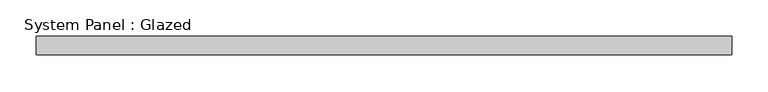
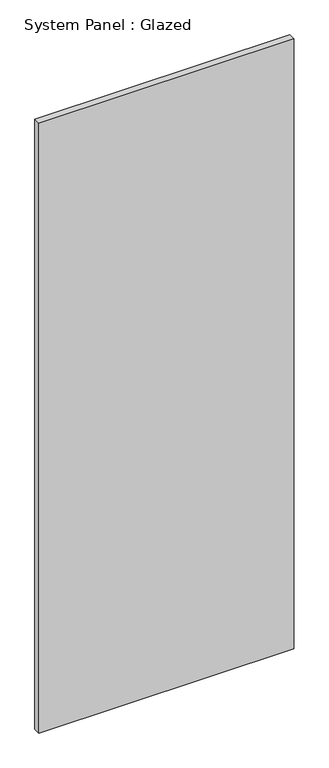
"""IFC4 building model written with IfcOpenShell, lengths in millimetres: plate geometry, System Panel : Glazed."""

from ifc_helpers import new_model, si_unit, origin, origin_with_axes, place, context, project, spatial, polyline, outline, extrude, source, transform, mapped, element, save


def system_panel_glazed_5a718088(model_context):
    return source(origin(), model_context, "Body", "SweptSolid", [
        extrude(outline(polyline([(477.3083333, 19.05), (-477.3083333, 19.05), (-477.3083333, 44.45), (477.3083333, 44.45), (477.3083333, 19.05)])), origin_with_axes(), (0.0, 0.0, 1.0), 2413.0),
    ])


if __name__ == "__main__":
    model = new_model("IFC4")
    model_context = context("Model", 3, world=origin())
    ifc_project = project(units=[si_unit("LENGTHUNIT", "METRE", prefix="MILLI")], contexts=[model_context])
    site = spatial("IfcSite", under=ifc_project)
    building = spatial("IfcBuilding", under=site)
    placement = place(None, origin())
    system_panel_glazed_shape = system_panel_glazed_5a718088(model_context)
    element("IfcPlate", 1, ObjectType="System Panel : Glazed", at=placement, inside=building, context=model_context, shape_type="MappedRepresentation", body=[
        mapped(system_panel_glazed_shape, transform((0.0, 0.0, 0.0), x_axis=(1.0, 0.0, 0.0), y_axis=(0.0, 1.0, 0.0), z_axis=(0.0, 0.0, 1.0))),
    ])
    save(model, "model.ifc")

# Revit data of these elements
# Type "System Panel : Glazed"
#   Construction Type Id = "GSP4R"
#   Analytic Construction = "1/8 in Pilkington single glazing"
#   Visual Light Transmittance = 0.9
#   Solar Heat Gain Coefficient = 0.86
#   Heat Transfer Coefficient (U) = 1.18115 BTU/(h·ft²·°F)
# Element 1 (IfcPlate, "System Panel : Glazed")
#   Materials on its faces: "Glass"
# Materials
#   "Glass": class "Glass", colour RGB 0 128 192, transparency 0.75, Description = "Soda Lime Glass", Cost = 0
